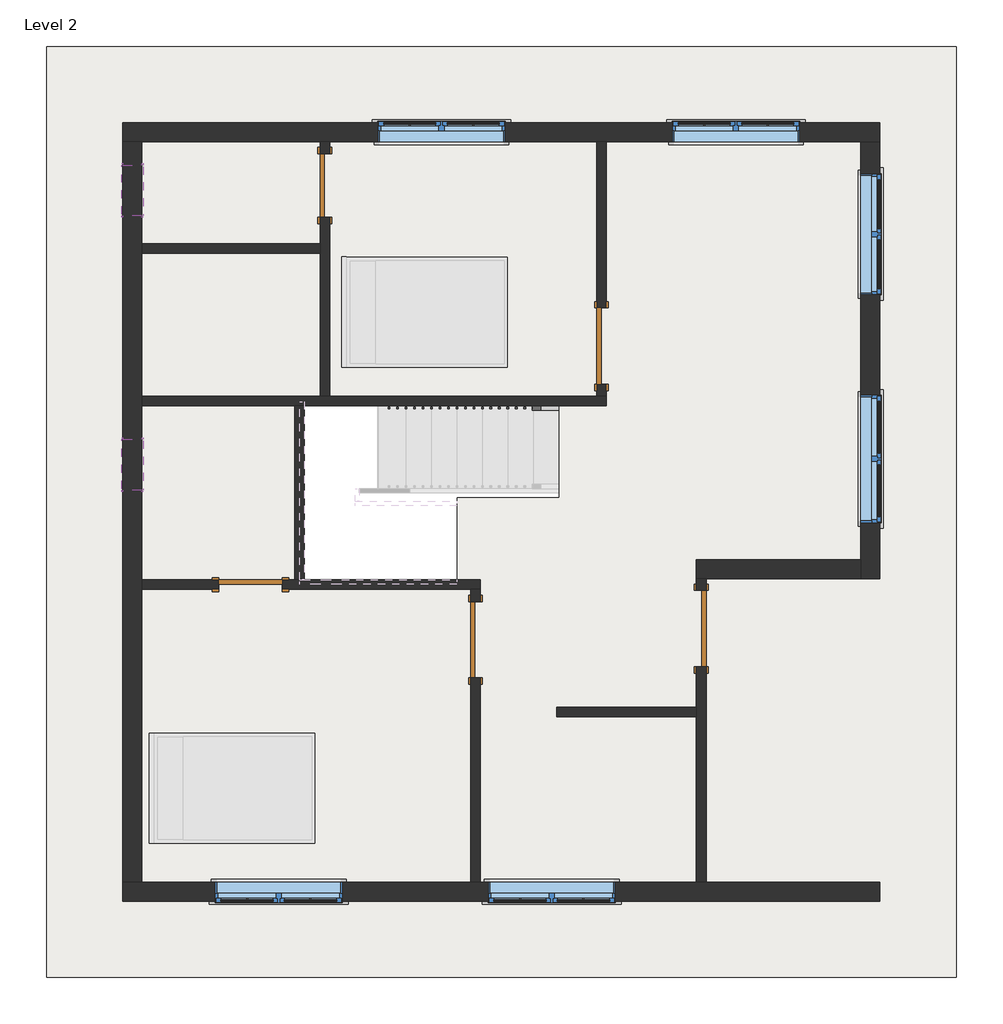
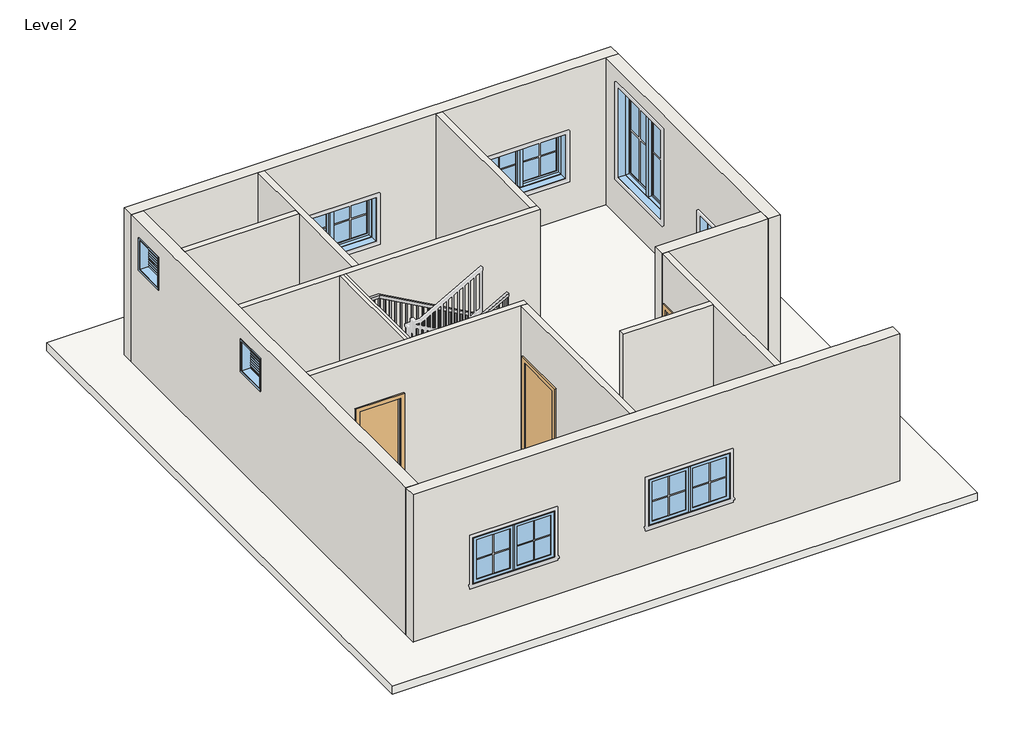
# One storey, part 1 of 2: 14 walls, 8 windows, 5 doors, 1 railing, 1 roof.
# Revit data of these elements (continued)
# Element 23 (IfcWindow, "Window-Casement-Double : WINDOW 6\"") (continued)
#   Exterior Wall Closure = 0' - 1 1/4"
#   Interior Trim Visibility = yes
#   Exterior Trim Visibility = yes
#   Phase Created = New Construction
#   Materials on its faces: "Wood - Stained", "Glass", "Clad - White"
# Element 24 (IfcWindow, "Window-Casement-Double : WINDOW 6\"")
#   Mark = "10"
#   Window Inset = 0' - 0"
#   Interior Wall Closure = 0' - 2 1/4"
#   Frame Extension = 0' - 0 1/4"
#   Exterior Wall Closure = 0' - 1 1/4"
#   Interior Trim Visibility = yes
#   Exterior Trim Visibility = yes
#   Phase Created = New Construction
#   Materials on its faces: "Wood - Stained", "Glass", "Clad - White"
# Element 25 (IfcWindow, "Window-Casement-Double : WINDOW 6\"")
#   Mark = "11"
#   Window Inset = 0' - 0"
#   Interior Wall Closure = 0' - 2 1/4"
#   Frame Extension = 0' - 0 1/4"
#   Exterior Wall Closure = 0' - 1 1/4"
#   Interior Trim Visibility = yes
#   Exterior Trim Visibility = yes
#   Phase Created = New Construction
#   Materials on its faces: "Wood - Stained", "Glass", "Clad - White"
# Element 26 (IfcWindow, "Window-Casement-Double : WINDOW 6\"")
#   Mark = "12"
#   Window Inset = 0' - 0"
#   Interior Wall Closure = 0' - 2 1/4"
#   Frame Extension = 0' - 0 1/4"
#   Exterior Wall Closure = 0' - 1 1/4"
#   Interior Trim Visibility = yes
#   Exterior Trim Visibility = yes
#   Phase Created = New Construction
#   Materials on its faces: "Wood - Stained", "Glass", "Clad - White"
# Element 27 (IfcWindow, "Window-Casement-Double : WINDOW 6\"")
#   Mark = "13"
#   Window Inset = 0' - 0"
#   Interior Wall Closure = 0' - 2 1/4"
#   Frame Extension = 0' - 0 1/4"
#   Exterior Wall Closure = 0' - 1 1/4"
#   Interior Trim Visibility = yes
#   Exterior Trim Visibility = yes
#   Phase Created = New Construction
#   Materials on its faces: "Wood - Stained", "Glass", "Clad - White"
# Element 28 (IfcWindow, "Window-Louvers : 24\" x 24\"")
#   Mark = "14"
#   Blade Width = 1' - 10 1/2"
#   Phase Created = New Construction
#   Materials on its faces: "Birch"
# Element 29 (IfcWindow, "Window-Louvers : 24\" x 24\"")
#   Mark = "15"
#   Blade Width = 1' - 10 1/2"
#   Phase Created = New Construction
#   Materials on its faces: "Birch"
# Materials
#   "Door - Panel": class "Wood", colour RGB 210 159 95, transparency 0, Cost = 0
#   "Door - Frame": colour RGB 118 70 51, transparency 0, Cost = 0
#   "Wood - Stained": class "Wood", colour RGB 224 178 126, transparency 0, Cost = 0
#   "Glass": class "Glass", colour RGB 0 128 192, transparency 0.75, Description = "Soda Lime Glass", Cost = 0
#   "Clad - White": class "Wood", colour RGB 242 242 238, transparency 0, Cost = 0
#   "Birch": class "Wood", colour RGB 224 178 126, transparency 0, Description = "Betula Alleghaniensis", Cost = 0
#   "Default Wall": colour RGB 128 128 128, transparency 0, Cost = 0
